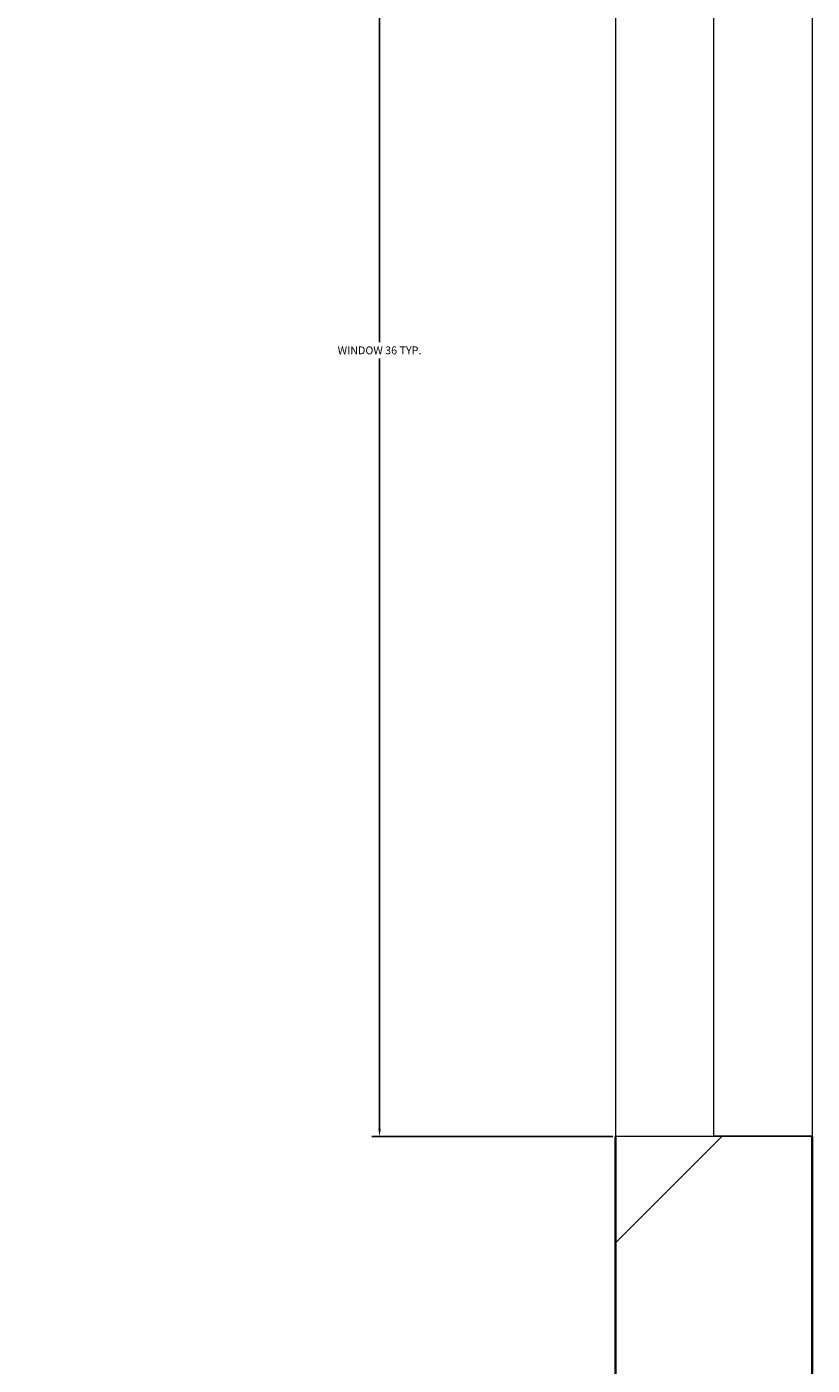
# Model space of a CAD drawing. Units: inches. Extents: x 2168 to 3056, y 1130 to 2629.
# Tile 18 of 42: x 2846 to 2864, y 2017 to 2048. Entities that reach past the tile are written whole.
import ezdxf

# ---------------------------------------------------------------- set-up
doc = ezdxf.new("R2010")
doc.units = ezdxf.units.IN
for name, color, linetype, lineweight in [('A-ANNO-DIMS', 2, 'Continuous', 18), ('A-GLAZ', 201, 'Continuous', 18), ('A-WALL', 7, 'Continuous', 35)]:
    doc.layers.add(name, color=color, linetype=linetype, lineweight=lineweight)
doc.layers.add('A-WALL-PATT', color=143, linetype='Continuous', lineweight=13, true_color=0x7aafdf)
doc.styles.get("Standard").update_dxf_attribs({"font": 'arial.ttf'})
doc.dimstyles.get("Standard").update_dxf_attribs({"dimtxt": 0.18, "dimasz": 0.18, "dimexe": 0.18, "dimexo": 0.0625, "dimgap": 0.09, "dimtad": 0, "dimtih": 1, "dimtoh": 1, "dimdec": 4, "dimzin": 0, "dimdsep": 46, "dimtxsty": 'Standard', "dimcen": 0.09, "dimadec": 0, "dimazin": 0, "dimtfac": 1, "dimtdec": 4, "dimtofl": 0, "dimtmove": 0, "dimatfit": 3, "dimfxl": 1, "dimtolj": 1, "dimtzin": 0, "dimarcsym": 0})

# ---------------------------------------------------------------- blocks, each defined once
blk = doc.blocks.new('WIN-36')
for p, q in [((0, 36), (0, 0)), ((2.25, 0), (2.25, 36)), ((4.5, 36), (4.5, 0)), ((0, 0), (4.5, 0)), ((4.5, 0), (2.25, 0))]:
    blk.add_line(p, q)
blk = doc.blocks.new('*D36')
at = {"layer": 'A-ANNO-DIMS', "color": 0, "lineweight": -2, "transparency": 16777216}
for p, q in [((2859.733, 2058.577), (2854.216, 2058.577)), ((2854.396, 2058.397), (2854.396, 2040.761)), ((2854.396, 2022.757), (2854.396, 2040.394)), ((2859.733, 2022.577), (2854.216, 2022.577))]:
    blk.add_line(p, q, dxfattribs=at)
at = {"layer": 'A-ANNO-DIMS', "color": 0, "transparency": 16777216}
for points in [[(2854.366, 2058.397), (2854.426, 2058.397), (2854.396, 2058.577)], [(2854.366, 2022.757), (2854.426, 2022.757), (2854.396, 2022.577)]]:
    blk.add_solid(points, dxfattribs=at)
at = {"layer": 'Defpoints', "color": 0, "transparency": 16777216}
for p in [(2854.396, 2058.577), (2859.796, 2058.577), (2859.796, 2022.577)]:
    blk.add_point(p, dxfattribs=at)
at = {"layer": 'A-ANNO-DIMS', "color": 0, "transparency": 16777216, "insert": (2854.396, 2040.577), "char_height": 0.18, "attachment_point": 5}
blk.add_mtext('\\A1;WINDOW 36 TYP.', dxfattribs=at)

msp = doc.modelspace()

# ---------------------------------------------------------------- hatches: boundary and pattern name
at = {"layer": 'A-WALL-PATT'}
h = msp.add_hatch(dxfattribs=at)
h.set_pattern_fill('ANSI32', color=256)
h.paths.add_polyline_path([(2463.796, 2409.389), (2467.387, 2409.389), (2467.387, 2413.889), (2454.768, 2413.889), (2454.768, 2411.639), (2454.768, 2409.389), (2459.296, 2409.389), (2459.296, 2265.389), (2455.644, 2265.389), (2455.644, 2260.889), (2467.349, 2260.889), (2467.349, 2263.139), (2467.349, 2265.389), (2463.796, 2265.389)])
h.paths.add_polyline_path([(2431.596, 2413.889), (2409.647, 2413.889), (2409.647, 2409.389), (2431.596, 2409.389), (2431.596, 2411.639)])
h.paths.add_polyline_path([(2349.647, 2413.889), (2331.796, 2413.889), (2331.796, 2362.671), (2336.296, 2362.671), (2336.296, 2409.389), (2349.647, 2409.389), (2349.647, 2411.639)])
h.paths.add_polyline_path([(2634.149, 2411.639), (2634.149, 2413.889), (2562.293, 2413.889), (2562.293, 2409.389), (2595.796, 2409.389), (2595.796, 2280.309), (2595.826, 2280.309), (2595.826, 2265.389), (2499.91, 2265.389), (2499.91, 2260.889), (2550.796, 2260.889), (2550.796, 2117.308), (2555.296, 2117.308), (2555.296, 2168.08), (2571.93, 2168.08), (2571.93, 2176.889), (2559.796, 2176.889), (2559.796, 2256.389), (2640.796, 2256.389), (2640.796, 2176.889), (2626.428, 2176.889), (2626.428, 2168.08), (2645.296, 2168.08), (2645.296, 2116.637), (2649.796, 2116.637), (2649.796, 2260.889), (2691.251, 2260.889), (2691.251, 2263.139), (2691.251, 2265.389), (2670.655, 2265.389), (2670.655, 2265.365), (2600.296, 2265.365), (2600.296, 2280.258), (2600.296, 2409.389), (2634.149, 2409.389)])
h.paths.add_polyline_path([(2600.296, 2473.889), (2612.84, 2473.889), (2612.84, 2478.389), (2572.636, 2478.389), (2572.636, 2473.889), (2595.796, 2473.889), (2595.796, 2413.889), (2600.296, 2413.889)])
h.paths.add_polyline_path([(2535.796, 2473.889), (2548.636, 2473.889), (2548.636, 2478.389), (2531.396, 2478.389), (2531.396, 2413.889), (2521.6, 2413.889), (2521.6, 2409.389), (2539.239, 2409.389), (2539.239, 2411.639), (2539.239, 2413.889), (2535.796, 2413.889)])
h.paths.add_polyline_path([(2664.796, 2478.389), (2636.84, 2478.389), (2636.84, 2473.889), (2660.296, 2473.889), (2660.296, 2413.889), (2656.165, 2413.889), (2656.165, 2409.389), (2671.684, 2409.389), (2671.684, 2411.639), (2671.684, 2413.889), (2664.796, 2413.889)])
h.paths.add_polyline_path([(2705.942, 2413.889), (2695.684, 2413.889), (2695.684, 2409.389), (2705.942, 2409.389)])
h.paths.add_polyline_path([(2741.35, 2413.889), (2728.733, 2413.889), (2728.733, 2411.639), (2728.733, 2409.389), (2732.296, 2409.389), (2732.296, 2265.389), (2725.733, 2265.389), (2725.733, 2260.889), (2740.917, 2260.889), (2740.917, 2263.139), (2740.917, 2265.389), (2736.796, 2265.389), (2736.796, 2409.389), (2741.35, 2409.389)])
h.paths.add_polyline_path([(2785.655, 2413.889), (2764.546, 2413.889), (2764.486, 2409.389), (2785.655, 2409.389), (2785.655, 2411.639)])
h.paths.add_polyline_path([(2864.296, 2413.889), (2845.655, 2413.889), (2845.655, 2409.389), (2859.796, 2409.389), (2859.796, 2368.425), (2864.296, 2368.425)])
h.paths.add_polyline_path([(2864.296, 2308.425), (2862.046, 2308.425), (2859.796, 2308.425), (2859.796, 2265.389), (2774.483, 2265.389), (2774.483, 2263.139), (2774.483, 2260.889), (2781.796, 2260.889), (2781.796, 2226.654), (2786.296, 2226.654), (2786.296, 2260.889), (2859.796, 2260.889), (2859.796, 2241.352), (2864.296, 2241.352)])
h.paths.add_polyline_path([(2864.296, 2217.352), (2862.046, 2217.352), (2859.796, 2217.352), (2859.796, 2200.889), (2786.296, 2200.889), (2786.296, 2205.931), (2784.046, 2205.931), (2781.796, 2205.931), (2781.796, 2150.974), (2786.296, 2150.974), (2786.296, 2161.889), (2859.796, 2161.889), (2859.796, 2144.419), (2864.296, 2144.419)])
h.paths.add_polyline_path([(2859.796, 2196.389), (2859.796, 2166.389), (2786.296, 2166.389), (2786.296, 2196.389)], flags=16)
h.paths.add_polyline_path([(2864.296, 2108.419), (2862.046, 2108.419), (2859.796, 2108.419), (2859.796, 2080.889), (2786.296, 2080.889), (2786.296, 2111.993), (2781.796, 2111.993), (2781.796, 2080.889), (2649.796, 2080.889), (2649.796, 2086.036), (2647.546, 2086.036), (2645.296, 2086.036), (2645.296, 2071.739), (2649.796, 2071.739), (2649.796, 2076.389), (2781.796, 2076.389), (2781.796, 2041.792), (2786.296, 2041.792), (2786.296, 2076.389), (2859.796, 2076.389), (2859.796, 2058.577), (2864.296, 2058.577)])
h.paths.add_polyline_path([(2864.296, 2022.577), (2859.796, 2022.577), (2859.796, 1992.389), (2786.296, 1992.389), (2786.296, 1999.573), (2781.796, 1999.573), (2781.796, 1848.085), (2784.046, 1848.085), (2786.296, 1848.085), (2786.296, 1851.389), (2859.796, 1851.389), (2859.796, 1838.258), (2864.296, 1838.258)], flags=17)
h.paths.add_polyline_path([(2859.796, 1987.889), (2859.796, 1855.889), (2786.296, 1855.889), (2786.296, 1987.889)], flags=16)
h.paths.add_polyline_path([(2823.046, 1987.889), (2841.421, 1921.889), (2823.046, 1855.889)], flags=0)
h.paths.add_polyline_path([(2864.296, 1814.258), (2859.796, 1814.258), (2859.796, 1791.389), (2786.296, 1791.389), (2786.296, 1825.658), (2784.046, 1825.658), (2781.796, 1825.658), (2781.796, 1791.389), (2720.155, 1791.389), (2720.155, 1791.265), (2649.796, 1791.265), (2649.796, 1806.159), (2649.796, 2038.983), (2647.546, 2038.983), (2645.296, 2038.983), (2645.296, 1783.925), (2649.796, 1783.925), (2649.796, 1786.889), (2781.796, 1786.889), (2781.796, 1746.789), (2786.296, 1746.789), (2786.296, 1786.889), (2859.796, 1786.889), (2859.796, 1770.083), (2864.296, 1770.083)])
h.paths.add_polyline_path([(2864.296, 1734.083), (2862.046, 1734.083), (2859.796, 1734.083), (2859.796, 1705.889), (2786.296, 1705.889), (2786.296, 1714.166), (2781.796, 1714.166), (2781.796, 1660.527), (2786.296, 1660.527), (2786.296, 1666.889), (2859.796, 1666.889), (2859.796, 1648.342), (2864.296, 1648.342)])
h.paths.add_polyline_path([(2786.296, 1701.389), (2859.796, 1701.389), (2859.796, 1671.389), (2786.296, 1671.389)], flags=16)
h.paths.add_polyline_path([(2649.796, 1756.576), (2647.546, 1756.576), (2645.296, 1756.576), (2645.296, 1606.889), (2555.296, 1606.889), (2555.296, 1749.513), (2553.046, 1749.513), (2550.796, 1749.513), (2550.796, 1606.889), (2503.006, 1606.889), (2503.006, 1604.639), (2503.006, 1602.389), (2595.796, 1602.389), (2595.849, 1602.389), (2595.849, 1587.495), (2595.796, 1458.389), (2561.502, 1458.389), (2561.502, 1456.139), (2561.502, 1453.889), (2595.796, 1453.889), (2595.796, 1381.889), (2573.438, 1381.889), (2573.438, 1377.389), (2613.01, 1377.389), (2613.01, 1379.639), (2613.01, 1381.889), (2600.296, 1381.889), (2600.296, 1453.889), (2634.327, 1453.889), (2634.327, 1458.389), (2600.296, 1458.389), (2600.296, 1602.389), (2670.655, 1602.389), (2694.095, 1602.389), (2694.095, 1606.889), (2649.796, 1606.889)])
h.paths.add_polyline_path([(2736.796, 1602.389), (2741.562, 1602.389), (2741.562, 1606.889), (2726.203, 1606.889), (2726.203, 1604.639), (2726.203, 1602.389), (2732.296, 1602.389), (2732.296, 1458.389), (2727.899, 1458.389), (2727.899, 1453.889), (2740.821, 1453.889), (2740.821, 1456.139), (2740.821, 1458.389), (2736.796, 1458.389)])
h.paths.add_polyline_path([(2859.796, 1606.889), (2786.296, 1606.889), (2786.296, 1637.334), (2784.046, 1637.334), (2781.796, 1637.334), (2781.796, 1606.889), (2775.612, 1606.889), (2775.612, 1602.389), (2859.796, 1602.389)])
h.paths.add_polyline_path([(2864.296, 1624.342), (2862.046, 1624.342), (2859.796, 1624.342), (2859.796, 1570.39), (2864.296, 1570.39)])
h.paths.add_polyline_path([(2864.296, 1510.39), (2862.046, 1510.39), (2859.796, 1510.39), (2859.796, 1458.389), (2846.735, 1458.389), (2846.735, 1456.139), (2846.735, 1453.889), (2864.296, 1453.889)])
h.paths.add_polyline_path([(2786.735, 1458.389), (2765.444, 1458.389), (2765.444, 1453.889), (2786.735, 1453.889)])
h.paths.add_polyline_path([(2706.004, 1458.389), (2695.36, 1458.389), (2695.36, 1453.889), (2706.004, 1453.889), (2706.004, 1456.139)])
h.paths.add_polyline_path([(2671.36, 1456.139), (2671.36, 1458.389), (2655.986, 1458.389), (2655.986, 1456.139), (2655.986, 1453.889), (2660.296, 1453.889), (2660.296, 1381.889), (2637.01, 1381.889), (2637.01, 1377.389), (2664.796, 1377.389), (2664.796, 1453.889), (2671.36, 1453.889)], flags=17)
h.paths.add_polyline_path([(2539.829, 1458.389), (2520.237, 1458.389), (2520.237, 1453.889), (2531.296, 1453.889), (2531.296, 1377.389), (2546.449, 1377.389), (2546.449, 1379.639), (2546.449, 1381.889), (2535.796, 1381.889), (2535.796, 1453.889), (2539.829, 1453.889)], flags=17)
h.paths.add_polyline_path([(2496.237, 1458.389), (2489.13, 1458.389), (2489.13, 1453.889), (2496.237, 1453.889), (2496.237, 1456.139)])
h.paths.add_polyline_path([(2467.433, 1456.139), (2467.433, 1458.389), (2463.796, 1458.389), (2463.796, 1602.389), (2468.242, 1602.389), (2468.242, 1605.7), (2468.242, 1606.889), (2454.602, 1606.889), (2454.602, 1602.389), (2459.296, 1602.389), (2459.296, 1458.389), (2454.24, 1458.389), (2454.24, 1453.889), (2467.433, 1453.889)])
h.paths.add_polyline_path([(2431.601, 1456.139), (2431.601, 1458.389), (2411.386, 1458.389), (2411.386, 1453.889), (2431.601, 1453.889)])
h.paths.add_polyline_path([(2351.386, 1458.389), (2336.296, 1458.389), (2336.296, 1490.693), (2334.046, 1490.693), (2331.796, 1490.693), (2331.796, 1453.889), (2351.386, 1453.889), (2351.386, 1456.139)])
h.paths.add_polyline_path([(2336.296, 1629.705), (2331.796, 1629.705), (2331.796, 1552.317), (2336.296, 1552.317), (2336.296, 1602.389), (2406.655, 1602.389), (2423.472, 1602.389), (2423.472, 1606.889), (2418.796, 1606.889), (2418.796, 1643.678), (2416.546, 1643.678), (2414.296, 1643.678), (2414.296, 1606.889), (2336.296, 1606.889)])
h.paths.add_polyline_path([(2418.796, 1714.384), (2414.296, 1714.384), (2414.296, 1705.889), (2336.296, 1705.889), (2336.296, 1731.324), (2334.046, 1731.324), (2331.796, 1731.324), (2331.796, 1653.705), (2334.046, 1653.705), (2336.296, 1653.705), (2336.296, 1666.889), (2414.296, 1666.889), (2414.296, 1663.589), (2418.796, 1663.589)])
h.paths.add_polyline_path([(2336.296, 1701.389), (2414.296, 1701.389), (2414.296, 1671.389), (2336.296, 1671.389)], flags=16)
h.paths.add_polyline_path([(2555.296, 2040.059), (2550.796, 2040.059), (2550.796, 1791.389), (2550.561, 1791.205), (2480.202, 1791.205), (2418.796, 1791.389), (2418.796, 1825.448), (2416.546, 1825.448), (2414.296, 1825.448), (2414.296, 1791.389), (2336.296, 1791.389), (2336.296, 1806.409), (2331.796, 1806.409), (2331.796, 1767.324), (2336.296, 1767.324), (2336.296, 1786.889), (2414.296, 1786.889), (2414.296, 1745.457), (2418.796, 1745.457), (2418.796, 1786.889), (2550.796, 1786.889), (2550.796, 1783.011), (2555.296, 1783.011)])
h.paths.add_polyline_path([(2418.796, 1923.389), (2423.207, 1923.389), (2423.207, 1925.639), (2423.207, 1927.889), (2418.796, 1927.889), (2418.796, 2000.048), (2414.296, 2000.048), (2414.296, 1992.389), (2336.296, 1992.389), (2336.296, 1987.889), (2414.296, 1987.889), (2414.296, 1855.889), (2336.296, 1855.889), (2336.296, 1851.389), (2414.296, 1851.389), (2414.296, 1846.759), (2418.796, 1846.759)], flags=17)
h.paths.add_polyline_path([(2336.296, 2019.294), (2334.046, 2019.294), (2331.796, 2019.294), (2331.796, 1830.409), (2336.296, 1830.409)], flags=17)
h.paths.add_polyline_path([(2550.796, 1927.889), (2453.541, 1927.889), (2453.541, 1925.639), (2453.541, 1923.389), (2550.796, 1923.389)], flags=17)
h.paths.add_polyline_path([(2744.987, 1927.889), (2649.796, 1927.889), (2649.796, 1923.389), (2744.987, 1923.389), (2744.987, 1925.639)], flags=17)
h.paths.add_polyline_path([(2555.296, 2086.458), (2553.046, 2086.458), (2550.796, 2086.458), (2550.796, 2080.889), (2418.796, 2080.889), (2336.296, 2080.889), (2336.296, 2115.399), (2334.046, 2115.399), (2331.796, 2115.399), (2331.796, 2055.294), (2336.296, 2055.294), (2336.296, 2076.389), (2550.796, 2076.389), (2550.796, 2071.538), (2555.296, 2071.538)])
h.paths.add_polyline_path([(2418.796, 2121.389), (2414.296, 2121.389), (2414.296, 2080.889), (2418.796, 2080.889)])
h.paths.add_polyline_path([(2418.796, 2076.389), (2414.296, 2076.389), (2414.296, 2035.123), (2418.796, 2035.123)])
h.paths.add_polyline_path([(2422.868, 2263.139), (2422.868, 2265.389), (2406.655, 2265.389), (2406.655, 2265.359), (2336.296, 2265.359), (2336.296, 2280.252), (2336.296, 2302.671), (2334.046, 2302.671), (2331.796, 2302.671), (2331.796, 2246.853), (2336.296, 2246.853), (2336.296, 2260.889), (2414.296, 2260.889), (2414.296, 2223.996), (2418.796, 2223.996), (2418.796, 2260.889), (2422.868, 2260.889)])
h.paths.add_polyline_path([(2418.796, 2204.783), (2416.546, 2204.783), (2414.296, 2204.783), (2414.296, 2200.889), (2336.296, 2200.889), (2336.296, 2220.853), (2331.796, 2220.853), (2331.796, 2151.399), (2336.296, 2151.399), (2336.296, 2161.889), (2414.296, 2161.889), (2414.296, 2153.726), (2418.796, 2153.726)])
h.paths.add_polyline_path([(2414.296, 2196.389), (2414.296, 2166.389), (2336.296, 2166.389), (2336.296, 2196.389)], flags=16)
h.paths.add_polyline_path([(2375.296, 2181.389), (2336.296, 2166.389), (2336.296, 2196.389)], flags=0)
h.paths.add_polyline_path([(2809.595, 2172.34), (2838.804, 2172.34), (2838.804, 2190.997), (2809.595, 2190.997)], flags=8)
h.paths.add_polyline_path([(2849.75, 1919.585), (2849.75, 1952.672), (2831.093, 1952.672), (2831.093, 1919.585)], flags=8)
h.paths.add_polyline_path([(2808.875, 1901.967), (2808.875, 1937.85), (2790.149, 1937.85), (2790.149, 1901.967)], flags=8)
h.paths.add_polyline_path([(2806.285, 1671.896), (2835.493, 1671.896), (2835.493, 1690.553), (2806.285, 1690.553)], flags=8)
h.paths.add_polyline_path([(2353.186, 1676.549), (2382.395, 1676.549), (2382.395, 1695.207), (2353.186, 1695.207)], flags=8)
h.paths.add_polyline_path([(2360.083, 1832.308), (2389.241, 1832.308), (2389.241, 1850.966), (2360.083, 1850.966)], flags=25)
h.paths.add_polyline_path([(2354.822, 2167.823), (2384.031, 2167.823), (2384.031, 2186.481), (2354.822, 2186.481)], flags=8)

# ---------------------------------------------------------------- linework, layer by layer
at = {"layer": 'A-GLAZ'}
msp.add_line((2864.296, 2022.577), (2864.296, 2022.577), dxfattribs=at)
at = {"layer": 'A-WALL'}
for p, q in [((2859.796, 2022.577), (2859.796, 1992.389)), ((2864.296, 2022.577), (2864.296, 1838.258))]:
    msp.add_line(p, q, dxfattribs=at)

# ---------------------------------------------------------------- block references
at = {"layer": 'A-GLAZ'}
msp.add_blockref('WIN-36', (2859.796, 2022.578), dxfattribs=at)

# ---------------------------------------------------------------- dimensions: what is measured, and where the dimension line sits
at = {"layer": 'A-ANNO-DIMS'}
dim = msp.add_linear_dim(base=(2854.396, 2058.577), p1=(2859.796, 2022.577), p2=(2859.796, 2058.577), angle=90, text='WINDOW <> TYP.', dimstyle='Standard', override={"dimdec": 0, "dimlfac": 1, "dimrnd": 0, "dimzin": 0, "dimdsep": 46, "dimlunit": 2}, dxfattribs=at)
dim.commit()
dim.dimension.update_dxf_attribs({"geometry": '*D36', "text_midpoint": (2854.396, 2040.577)})

doc.saveas('drawing.dxf')
